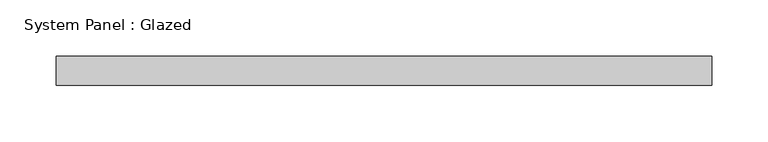
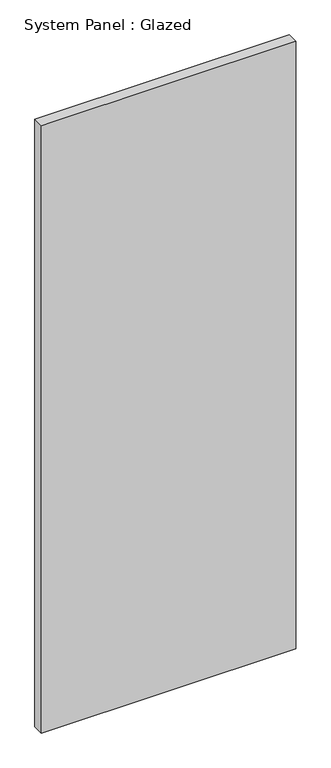
"""IFC4 building model written with IfcOpenShell, lengths in millimetres: plate geometry, System Panel : Glazed."""

from ifc_helpers import new_model, si_unit, origin, origin_with_axes, place, context, project, spatial, polyline, outline, extrude, source, transform, mapped, element, save


def system_panel_glazed_9cb0e95b(model_context):
    return source(origin(), model_context, "Body", "SweptSolid", [
        extrude(outline(polyline([(289.9833333, 19.05), (-289.9833333, 19.05), (-289.9833333, 44.45), (289.9833333, 44.45), (289.9833333, 19.05)])), origin_with_axes(), (0.0, 0.0, 1.0), 1463.48195),
    ])


if __name__ == "__main__":
    model = new_model("IFC4")
    model_context = context("Model", 3, world=origin())
    ifc_project = project(units=[si_unit("LENGTHUNIT", "METRE", prefix="MILLI")], contexts=[model_context])
    site = spatial("IfcSite", under=ifc_project)
    building = spatial("IfcBuilding", under=site)
    placement = place(None, origin())
    system_panel_glazed_shape = system_panel_glazed_9cb0e95b(model_context)
    element("IfcPlate", 1, ObjectType="System Panel : Glazed", at=placement, inside=building, context=model_context, shape_type="MappedRepresentation", body=[
        mapped(system_panel_glazed_shape, transform((0.0, 0.0, 0.0), x_axis=(1.0, 0.0, 0.0), y_axis=(0.0, 1.0, 0.0), z_axis=(0.0, 0.0, 1.0))),
    ])
    save(model, "model.ifc")

# Revit data of these elements
# Type "System Panel : Glazed"
#   Construction Type Id = "GSP4R"
#   Analytic Construction = "1/8 in Pilkington single glazing"
#   Visual Light Transmittance = 0.9
#   Solar Heat Gain Coefficient = 0.86
#   Heat Transfer Coefficient (U) = 1.18115 BTU/(h·ft²·°F)
# Element 1 (IfcPlate, "System Panel : Glazed")
#   Materials on its faces: "Glass"
# Materials
#   "Glass": class "Glass", colour RGB 0 128 192, transparency 0.75, Description = "Soda Lime Glass", Cost = 0
